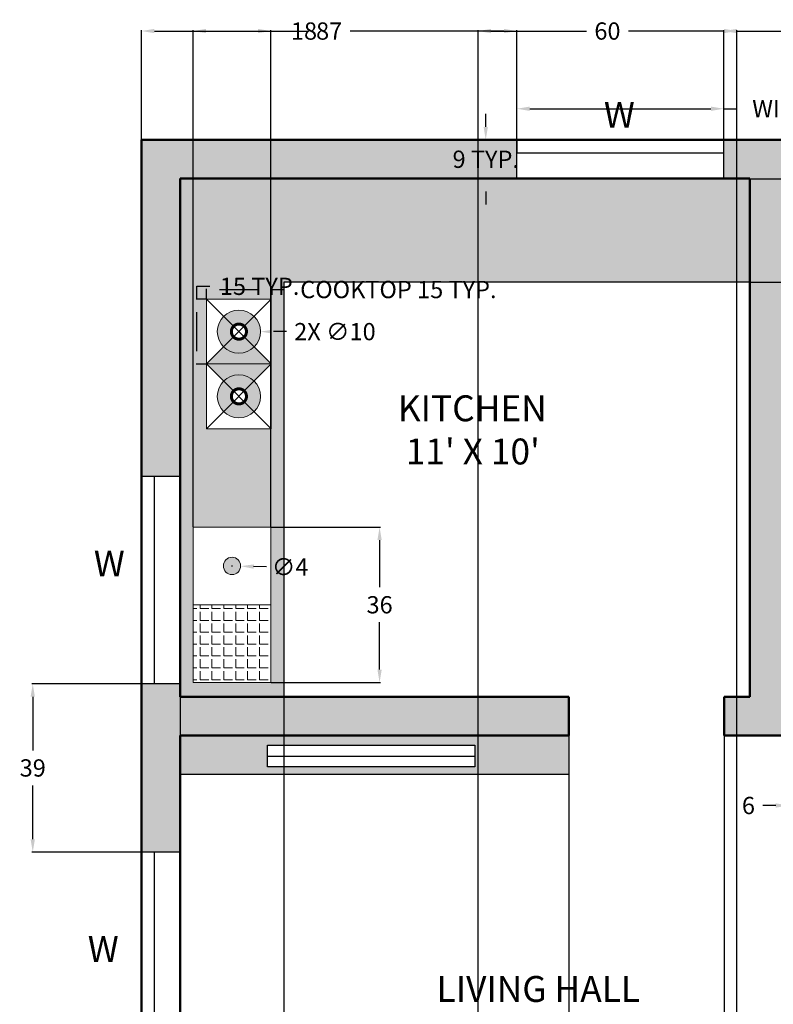
# Model space of a CAD drawing. Units: inches. Extents: x 30 to 385, y 81 to 626.
# Tile 3 of 4: x 30 to 204, y 398 to 626. Entities that reach past the tile are written whole.
import ezdxf

# ---------------------------------------------------------------- set-up
doc = ezdxf.new("R2010")
doc.units = ezdxf.units.IN
doc.header["$MEASUREMENT"] = 0
for name, color, linetype, lineweight in [('A-ANNO-DIMS', 2, 'Continuous', 18), ('A-ANNO-TEXT', 7, 'Continuous', 18), ('A-AREA-IDEN', 7, 'Continuous', 25), ('A-EQPM', 9, 'Continuous', 18), ('A-FLOR-CASE', 8, 'Continuous', 25), ('A-FLOR-CASE-PATT', 26, 'Continuous', 13), ('A-FLOR-FIXT', 8, 'Continuous', 18), ('A-FLOR-FIXT-PATT', 9, 'Continuous', 13), ('A-GLAZ', 4, 'Continuous', 25), ('A-WALL', 7, 'Continuous', 50), ('A-WALL-PATT', 32, 'Continuous', 13)]:
    doc.layers.add(name, color=color, linetype=linetype, lineweight=lineweight)
doc.styles.get("Standard").update_dxf_attribs({"font": 'arial.ttf'})
doc.dimstyles.get("Standard").update_dxf_attribs({"dimtxt": 4, "dimasz": 3, "dimexe": 0.18, "dimexo": 0.0625, "dimgap": 2, "dimtad": 0, "dimtih": 1, "dimtoh": 1, "dimdec": 0, "dimzin": 0, "dimdsep": 46, "dimlunit": 3, "dimtxsty": 'Standard', "dimcen": 0.09, "dimadec": 0, "dimazin": 0, "dimtfac": 1, "dimtdec": 0, "dimtofl": 0, "dimtmove": 0, "dimatfit": 3, "dimfxl": 1, "dimtolj": 1, "dimtzin": 0, "dimarcsym": 0})

# ---------------------------------------------------------------- blocks, each defined once
blk = doc.blocks.new('WIN-48')
for p, q in [((0, 0), (0, 9)), ((48, 0), (48, 9)), ((0, 6), (48, 6))]:
    blk.add_line(p, q)
blk = doc.blocks.new('COOKTOP-BURNER')
for p, q in [((-7.5, 7.5), (7.5, -7.5)), ((-7.5, -7.5), (7.5, 7.5))]:
    blk.add_line(p, q)
at = {"const_width": 0.7}
blk.add_lwpolyline([(-1.75, 0, 1), (1.75, 0, 1)], format="xyb", close=True, dxfattribs=at)
blk.add_circle((0, 0), 5)
blk = doc.blocks.new('*D6')
at = {"layer": 'A-ANNO-DIMS', "color": 0, "lineweight": -2, "transparency": 16777216}
for p, q in [((144.92, 598.13), (144.92, 605.44)), ((147.92, 605.26), (189.92, 605.26)), ((192.92, 598.13), (192.92, 605.44)), ((192.92, 605.26), (195.92, 605.26))]:
    blk.add_line(p, q, dxfattribs=at)
at = {"layer": 'A-ANNO-DIMS', "color": 0, "transparency": 16777216}
for points in [[(147.92, 605.76), (147.92, 604.76), (144.92, 605.26)], [(189.92, 605.76), (189.92, 604.76), (192.92, 605.26)]]:
    blk.add_solid(points, dxfattribs=at)
at = {"layer": 'Defpoints', "color": 0, "transparency": 16777216}
for p in [(192.92, 605.26), (144.92, 598.06), (192.92, 598.06)]:
    blk.add_point(p, dxfattribs=at)
at = {"layer": 'A-ANNO-DIMS', "color": 0, "transparency": 16777216, "insert": (220.77, 605.26), "char_height": 4, "attachment_point": 5}
blk.add_mtext('\\A1;WINDOW 48 TYP.', dxfattribs=at)
blk = doc.blocks.new('*D7')
at = {"layer": 'A-ANNO-DIMS', "color": 0, "lineweight": -2, "transparency": 16777216}
for p, q in [((137.72, 601.06), (137.72, 604.06)), ((144.86, 598.06), (137.54, 598.06)), ((144.86, 589.06), (137.54, 589.06)), ((137.72, 586.06), (137.72, 583.06))]:
    blk.add_line(p, q, dxfattribs=at)
at = {"layer": 'A-ANNO-DIMS', "color": 0, "transparency": 16777216}
for points in [[(137.22, 601.06), (138.22, 601.06), (137.72, 598.06)], [(137.22, 586.06), (138.22, 586.06), (137.72, 589.06)]]:
    blk.add_solid(points, dxfattribs=at)
at = {"layer": 'Defpoints', "color": 0, "transparency": 16777216}
for p in [(137.72, 598.06), (144.92, 598.06), (144.92, 589.06)]:
    blk.add_point(p, dxfattribs=at)
at = {"layer": 'A-ANNO-DIMS', "color": 0, "transparency": 16777216, "insert": (137.72, 593.56), "char_height": 4, "attachment_point": 5}
blk.add_mtext('\\A1;9 TYP.', dxfattribs=at)
blk = doc.blocks.new('*D14')
at = {"layer": 'A-ANNO-DIMS', "color": 0, "lineweight": -2, "transparency": 16777216}
for p, q in [((73, 561.2), (73, 563.56)), ((76, 563.38), (85, 563.38)), ((88, 561.2), (88, 563.56)), ((88, 563.38), (91, 563.38))]:
    blk.add_line(p, q, dxfattribs=at)
at = {"layer": 'A-ANNO-DIMS', "color": 0, "transparency": 16777216}
for points in [[(76, 563.88), (76, 562.88), (73, 563.38)], [(85, 563.88), (85, 562.88), (88, 563.38)]]:
    blk.add_solid(points, dxfattribs=at)
at = {"layer": 'Defpoints', "color": 0, "transparency": 16777216}
for p in [(88, 563.38), (73, 561.13), (88, 561.13)]:
    blk.add_point(p, dxfattribs=at)
at = {"layer": 'A-ANNO-DIMS', "color": 0, "transparency": 16777216, "insert": (117.46, 563.38), "char_height": 4, "attachment_point": 5}
blk.add_mtext('\\A1;COOKTOP 15 TYP.', dxfattribs=at)
blk = doc.blocks.new('*D15')
at = {"layer": 'A-ANNO-DIMS', "color": 0, "lineweight": -2, "transparency": 16777216}
for p, q in [((70.75, 561.13), (70.75, 564.13)), ((70.75, 564.13), (73.75, 564.13)), ((72.94, 561.13), (70.57, 561.13)), ((70.75, 549.13), (70.75, 558.13)), ((72.94, 546.13), (70.57, 546.13))]:
    blk.add_line(p, q, dxfattribs=at)
at = {"layer": 'A-ANNO-DIMS', "color": 0, "transparency": 16777216}
for points in [[(70.25, 558.13), (71.25, 558.13), (70.75, 561.13)], [(70.25, 549.13), (71.25, 549.13), (70.75, 546.13)]]:
    blk.add_solid(points, dxfattribs=at)
at = {"layer": 'Defpoints', "color": 0, "transparency": 16777216}
for p in [(70.75, 561.13), (73, 561.13), (73, 546.13)]:
    blk.add_point(p, dxfattribs=at)
at = {"layer": 'A-ANNO-DIMS', "color": 0, "transparency": 16777216, "insert": (85.3, 564.13), "char_height": 4, "attachment_point": 5}
blk.add_mtext('\\A1;15 TYP.', dxfattribs=at)
blk = doc.blocks.new('*D25')
at = {"layer": 'A-ANNO-DIMS', "color": 0, "lineweight": -2, "transparency": 16777216}
for p, q in [((57.86, 472.06), (32.54, 472.06)), ((32.72, 469.06), (32.72, 456.61)), ((32.72, 436.06), (32.72, 448.52)), ((57.86, 433.06), (32.54, 433.06))]:
    blk.add_line(p, q, dxfattribs=at)
at = {"layer": 'A-ANNO-DIMS', "color": 0, "transparency": 16777216}
for points in [[(32.22, 469.06), (33.22, 469.06), (32.72, 472.06)], [(32.22, 436.06), (33.22, 436.06), (32.72, 433.06)]]:
    blk.add_solid(points, dxfattribs=at)
at = {"layer": 'Defpoints', "color": 0, "transparency": 16777216}
for p in [(32.72, 472.06), (57.92, 472.06), (57.92, 433.06)]:
    blk.add_point(p, dxfattribs=at)
at = {"layer": 'A-ANNO-DIMS', "color": 0, "transparency": 16777216, "insert": (32.72, 452.56), "char_height": 4, "attachment_point": 5}
blk.add_mtext('\\A1;39', dxfattribs=at)
blk = doc.blocks.new('*D26')
at = {"layer": 'A-ANNO-DIMS', "color": 0, "lineweight": -2, "transparency": 16777216}
for p, q in [((57.92, 598.13), (57.92, 623.44)), ((60.92, 623.26), (96.55, 623.26)), ((141.92, 623.26), (106.29, 623.26)), ((144.92, 598.13), (144.92, 623.44))]:
    blk.add_line(p, q, dxfattribs=at)
at = {"layer": 'A-ANNO-DIMS', "color": 0, "transparency": 16777216}
for points in [[(60.92, 623.76), (60.92, 622.76), (57.92, 623.26)], [(141.92, 623.76), (141.92, 622.76), (144.92, 623.26)]]:
    blk.add_solid(points, dxfattribs=at)
at = {"layer": 'Defpoints', "color": 0, "transparency": 16777216}
for p in [(144.92, 623.26), (57.92, 598.06), (144.92, 598.06)]:
    blk.add_point(p, dxfattribs=at)
at = {"layer": 'A-ANNO-DIMS', "color": 0, "transparency": 16777216, "insert": (101.42, 623.26), "char_height": 4, "attachment_point": 5}
blk.add_mtext('\\A1;87', dxfattribs=at)
blk = doc.blocks.new('*D27')
at = {"layer": 'A-ANNO-DIMS', "color": 0, "lineweight": -2, "transparency": 16777216}
for p, q in [((192.92, 598.13), (192.92, 623.44)), ((195.92, 623.26), (207.92, 623.26)), ((210.92, 598.13), (210.92, 623.44)), ((210.92, 623.26), (213.92, 623.26))]:
    blk.add_line(p, q, dxfattribs=at)
at = {"layer": 'A-ANNO-DIMS', "color": 0, "transparency": 16777216}
for points in [[(195.92, 623.76), (195.92, 622.76), (192.92, 623.26)], [(207.92, 623.76), (207.92, 622.76), (210.92, 623.26)]]:
    blk.add_solid(points, dxfattribs=at)
at = {"layer": 'Defpoints', "color": 0, "transparency": 16777216}
for p in [(210.92, 623.26), (192.92, 598.06), (210.92, 598.06)]:
    blk.add_point(p, dxfattribs=at)
at = {"layer": 'A-ANNO-DIMS', "color": 0, "transparency": 16777216, "insert": (218.6, 623.26), "char_height": 4, "attachment_point": 5}
blk.add_mtext('\\A1;18', dxfattribs=at)
blk = doc.blocks.new('*D28')
at = {"layer": 'A-ANNO-DIMS', "color": 0, "lineweight": -2, "transparency": 16777216}
for p, q in [((66.92, 469), (66.92, 83.68)), ((90.92, 469), (90.92, 83.68)), ((69.92, 83.86), (74.03, 83.86)), ((87.92, 83.86), (83.81, 83.86))]:
    blk.add_line(p, q, dxfattribs=at)
at = {"layer": 'A-ANNO-DIMS', "color": 0, "transparency": 16777216}
for points in [[(69.92, 84.36), (69.92, 83.36), (66.92, 83.86)], [(87.92, 84.36), (87.92, 83.36), (90.92, 83.86)]]:
    blk.add_solid(points, dxfattribs=at)
at = {"layer": 'Defpoints', "color": 0, "transparency": 16777216}
for p in [(66.92, 469.06), (90.92, 469.06), (90.92, 83.86)]:
    blk.add_point(p, dxfattribs=at)
at = {"layer": 'A-ANNO-DIMS', "color": 0, "transparency": 16777216, "insert": (78.92, 83.86), "char_height": 4, "attachment_point": 5}
blk.add_mtext('\\A1;24', dxfattribs=at)
blk = doc.blocks.new('*D29')
at = {"layer": 'A-ANNO-DIMS', "color": 0, "lineweight": -2, "transparency": 16777216}
for p, q in [((198.98, 589.06), (374.3, 589.06)), ((374.12, 586.06), (374.12, 581.07)), ((374.12, 568.06), (374.12, 573.06)), ((198.98, 565.06), (374.3, 565.06))]:
    blk.add_line(p, q, dxfattribs=at)
at = {"layer": 'A-ANNO-DIMS', "color": 0, "transparency": 16777216}
for points in [[(373.62, 586.06), (374.62, 586.06), (374.12, 589.06)], [(373.62, 568.06), (374.62, 568.06), (374.12, 565.06)]]:
    blk.add_solid(points, dxfattribs=at)
at = {"layer": 'Defpoints', "color": 0, "transparency": 16777216}
for p in [(198.92, 589.06), (374.12, 589.06), (198.92, 565.06)]:
    blk.add_point(p, dxfattribs=at)
at = {"layer": 'A-ANNO-DIMS', "color": 0, "transparency": 16777216, "insert": (374.12, 577.06), "char_height": 4, "attachment_point": 5}
blk.add_mtext('\\A1;24', dxfattribs=at)
blk = doc.blocks.new('*D30')
at = {"layer": 'A-ANNO-DIMS', "color": 0, "lineweight": -2, "transparency": 16777216}
for p, q in [((69.91, 508.42), (69.91, 623.44)), ((72.91, 623.26), (84.91, 623.26)), ((87.91, 508.42), (87.91, 623.44)), ((87.91, 623.26), (90.91, 623.26))]:
    blk.add_line(p, q, dxfattribs=at)
at = {"layer": 'A-ANNO-DIMS', "color": 0, "transparency": 16777216}
for points in [[(72.91, 623.76), (72.91, 622.76), (69.91, 623.26)], [(84.91, 623.76), (84.91, 622.76), (87.91, 623.26)]]:
    blk.add_solid(points, dxfattribs=at)
at = {"layer": 'Defpoints', "color": 0, "transparency": 16777216}
for p in [(87.91, 623.26), (69.91, 508.36), (87.91, 508.36)]:
    blk.add_point(p, dxfattribs=at)
at = {"layer": 'A-ANNO-DIMS', "color": 0, "transparency": 16777216, "insert": (95.59, 623.26), "char_height": 4, "attachment_point": 5}
blk.add_mtext('\\A1;18', dxfattribs=at)
blk = doc.blocks.new('*D31')
at = {"layer": 'A-ANNO-DIMS', "color": 0, "lineweight": -2, "transparency": 16777216}
for p, q in [((87.97, 508.36), (113.29, 508.36)), ((113.11, 505.36), (113.11, 494.4)), ((113.11, 475.36), (113.11, 486.31)), ((87.97, 472.36), (113.29, 472.36))]:
    blk.add_line(p, q, dxfattribs=at)
at = {"layer": 'A-ANNO-DIMS', "color": 0, "transparency": 16777216}
for points in [[(112.61, 505.36), (113.61, 505.36), (113.11, 508.36)], [(112.61, 475.36), (113.61, 475.36), (113.11, 472.36)]]:
    blk.add_solid(points, dxfattribs=at)
at = {"layer": 'Defpoints', "color": 0, "transparency": 16777216}
for p in [(87.91, 508.36), (87.91, 472.36), (113.11, 472.36)]:
    blk.add_point(p, dxfattribs=at)
at = {"layer": 'A-ANNO-DIMS', "color": 0, "transparency": 16777216, "insert": (113.11, 490.36), "char_height": 4, "attachment_point": 5}
blk.add_mtext('\\A1;36', dxfattribs=at)
blk = doc.blocks.new('*D32')
at = {"layer": 'A-ANNO-DIMS', "color": 0, "lineweight": -2, "transparency": 16777216}
for p, q in [((135.92, 247.13), (135.92, 623.44)), ((138.92, 623.26), (161.05, 623.26)), ((192.92, 623.26), (170.79, 623.26)), ((195.92, 247.13), (195.92, 623.44))]:
    blk.add_line(p, q, dxfattribs=at)
at = {"layer": 'A-ANNO-DIMS', "color": 0, "transparency": 16777216}
for points in [[(138.92, 623.76), (138.92, 622.76), (135.92, 623.26)], [(192.92, 623.76), (192.92, 622.76), (195.92, 623.26)]]:
    blk.add_solid(points, dxfattribs=at)
at = {"layer": 'Defpoints', "color": 0, "transparency": 16777216}
for p in [(195.92, 623.26), (135.92, 247.06), (195.92, 247.06)]:
    blk.add_point(p, dxfattribs=at)
at = {"layer": 'A-ANNO-DIMS', "color": 0, "transparency": 16777216, "insert": (165.92, 623.26), "char_height": 4, "attachment_point": 5}
blk.add_mtext('\\A1;60', dxfattribs=at)
blk = doc.blocks.new('*D33')
at = {"layer": 'A-ANNO-DIMS', "color": 0, "lineweight": -2, "transparency": 16777216}
for p, q in [((156.96, 460), (156.96, 83.68)), ((192.96, 460), (192.96, 83.68)), ((159.96, 83.86), (170.09, 83.86)), ((189.96, 83.86), (179.82, 83.86))]:
    blk.add_line(p, q, dxfattribs=at)
at = {"layer": 'A-ANNO-DIMS', "color": 0, "transparency": 16777216}
for points in [[(159.96, 84.36), (159.96, 83.36), (156.96, 83.86)], [(189.96, 84.36), (189.96, 83.36), (192.96, 83.86)]]:
    blk.add_solid(points, dxfattribs=at)
at = {"layer": 'Defpoints', "color": 0, "transparency": 16777216}
for p in [(156.96, 460.06), (192.96, 460.06), (192.96, 83.86)]:
    blk.add_point(p, dxfattribs=at)
at = {"layer": 'A-ANNO-DIMS', "color": 0, "transparency": 16777216, "insert": (174.96, 83.86), "char_height": 4, "attachment_point": 5}
blk.add_mtext('\\A1;36', dxfattribs=at)
blk = doc.blocks.new('*D35')
at = {"layer": 'A-ANNO-DIMS', "color": 0, "lineweight": -2, "transparency": 16777216}
for p, q in [((207.92, 469), (207.92, 443.68)), ((213.92, 469), (213.92, 443.68)), ((204.92, 443.86), (201.92, 443.86)), ((216.92, 443.86), (219.92, 443.86))]:
    blk.add_line(p, q, dxfattribs=at)
at = {"layer": 'A-ANNO-DIMS', "color": 0, "transparency": 16777216}
for points in [[(204.92, 444.36), (204.92, 443.36), (207.92, 443.86)], [(216.92, 444.36), (216.92, 443.36), (213.92, 443.86)]]:
    blk.add_solid(points, dxfattribs=at)
at = {"layer": 'Defpoints', "color": 0, "transparency": 16777216}
for p in [(207.92, 469.06), (213.92, 469.06), (207.92, 443.86)]:
    blk.add_point(p, dxfattribs=at)
at = {"layer": 'A-ANNO-DIMS', "color": 0, "transparency": 16777216, "insert": (198.6, 443.86), "char_height": 4, "attachment_point": 5}
blk.add_mtext('\\A1;6', dxfattribs=at)
blk = doc.blocks.new('*D52')
at = {"layer": 'A-ANNO-DIMS', "color": 0, "lineweight": -2, "transparency": 16777216}
for p, q in [((78.82, 499.36), (79, 499.36)), ((78.91, 499.27), (78.91, 499.45)), ((86.9, 499.13), (83.9, 499.21))]:
    blk.add_line(p, q, dxfattribs=at)
at = {"layer": 'A-ANNO-DIMS', "color": 0, "transparency": 16777216}
blk.add_solid([(83.92, 499.71), (83.89, 498.71), (80.91, 499.3)], dxfattribs=at)
at = {"layer": 'Defpoints', "color": 0, "transparency": 16777216}
for p in [(76.91, 499.42), (80.91, 499.3)]:
    blk.add_point(p, dxfattribs=at)
at = {"layer": 'A-ANNO-DIMS', "color": 0, "transparency": 16777216, "insert": (92.38, 499.13), "char_height": 4, "attachment_point": 5}
blk.add_mtext('\\A1;∅4', dxfattribs=at)
blk = doc.blocks.new('*D53')
at = {"layer": 'A-ANNO-DIMS', "color": 0, "lineweight": -2, "transparency": 16777216}
for p, q in [((80.41, 553.63), (80.59, 553.63)), ((80.5, 553.54), (80.5, 553.72)), ((91.5, 553.63), (88.5, 553.63))]:
    blk.add_line(p, q, dxfattribs=at)
at = {"layer": 'A-ANNO-DIMS', "color": 0, "transparency": 16777216}
blk.add_solid([(88.5, 554.13), (88.5, 553.13), (85.5, 553.63)], dxfattribs=at)
at = {"layer": 'Defpoints', "color": 0, "transparency": 16777216}
for p in [(75.5, 553.63), (85.5, 553.63)]:
    blk.add_point(p, dxfattribs=at)
at = {"layer": 'A-ANNO-DIMS', "color": 0, "transparency": 16777216, "insert": (102.76, 553.63), "char_height": 4, "attachment_point": 5}
blk.add_mtext('\\A1;2X ∅10', dxfattribs=at)

msp = doc.modelspace()

# ---------------------------------------------------------------- hatches: boundary and pattern name
at = {"layer": 'A-FLOR-CASE-PATT'}
h = msp.add_hatch(color=256, dxfattribs=at)
h.paths.add_polyline_path([(198.919, 589.0638), (66.919, 589.0638), (66.919, 469.0638), (90.919, 469.0638), (90.919, 565.0638), (198.919, 565.0638)])
h.paths.add_polyline_path([(88.002, 561.1334), (88.002, 531.1334), (73.002, 531.1334), (73.002, 561.1334)], flags=16)
h.paths.add_polyline_path([(85.502, 553.6334, -0.19891237), (84.0375, 550.0979), (88.002, 546.1334), (84.0375, 542.1689, -0.19891237), (85.502, 538.6334, -1), (75.502, 538.6334, -0.19891237), (76.9665, 542.1689), (73.002, 546.1334), (76.9665, 550.0979, -0.19891237), (75.502, 553.6334, -1)], flags=0)
h.paths.add_polyline_path([(82.2476, 553.6334, -1), (78.7564, 553.6334, -1)], flags=0)
h.paths.add_polyline_path([(82.2476, 538.6334, -1), (78.7564, 538.6334, -1)], flags=0)
h.paths.add_polyline_path([(87.9068, 508.3581), (87.9068, 472.3581), (69.9068, 472.3581), (69.9068, 508.3581)], flags=16)
h.paths.add_polyline_path([(80.9068, 499.3581, -1), (76.9068, 499.3581, -1)], flags=0)
h = msp.add_hatch(color=256, dxfattribs=at)
h.paths.add_polyline_path([(156.9551, 460.0638), (66.919, 460.0638), (66.919, 451.0638), (156.9551, 451.0638)])
h.paths.add_polyline_path([(135.1556, 452.8), (87.1556, 452.8), (87.1556, 457.8), (135.1556, 457.8)], flags=16)
at = {"layer": 'A-FLOR-FIXT-PATT'}
h = msp.add_hatch(dxfattribs=at)
h.set_pattern_fill('ANGLE', color=256, scale=10)
h.set_pattern_definition([(0, (0, 0), (0, 2.75), [2, -0.75]), (90, (0, 0), (-2.75, 2e-16), [2, -0.75])])
h.paths.add_polyline_path([(87.9068, 490.3581), (69.9068, 490.3581), (69.9068, 472.3581), (87.9068, 472.3581)])
at = {"layer": 'A-WALL-PATT'}
msp.add_hatch(color=256, dxfattribs=at).paths.add_polyline_path([(144.919, 598.0638), (57.919, 598.0638), (57.919, 520.0638), (66.919, 520.0638), (66.919, 589.0638), (144.919, 589.0638)])
h = msp.add_hatch(color=256, dxfattribs=at)
h.paths.add_polyline_path([(156.9551, 469.0638), (66.919, 469.0638), (66.919, 472.0638), (57.919, 472.0638), (57.919, 433.0638), (66.919, 433.0638), (66.919, 460.0638), (156.9551, 460.0638)])
h.paths.add_polyline_path([(207.919, 589.0638), (210.919, 589.0638), (210.919, 598.0638), (192.919, 598.0638), (192.919, 589.0638), (198.919, 589.0638), (198.919, 469.0638), (192.9551, 469.0638), (192.9551, 460.0638), (213.919, 460.0638), (213.919, 469.0638), (207.919, 469.0638)])
h.paths.add_polyline_path([(348.919, 598.0638), (258.919, 598.0638), (258.919, 589.0638), (339.919, 589.0638), (339.919, 469.0638), (336.919, 469.0638), (336.919, 460.0638), (339.919, 460.0638), (339.919, 442.0638), (348.919, 442.0638)])

# ---------------------------------------------------------------- linework, layer by layer
at = {"layer": 'A-EQPM'}
for p, q in [((73.002, 546.1334), (88.002, 546.1334)), ((73.002, 531.1334), (88.002, 531.1334))]:
    msp.add_line(p, q, dxfattribs=at)
msp.add_lwpolyline([(73.002, 561.1334), (88.002, 561.1334), (88.002, 531.1334), (73.002, 531.1334)], close=True, dxfattribs=at)
at = {"layer": 'A-FLOR-CASE'}
for p, q in [((198.919, 565.0638), (90.919, 565.0638)), ((90.919, 565.0638), (90.919, 469.0638)), ((156.9551, 460.0638), (156.9551, 451.0638)), ((87.1556, 455.3), (135.1556, 455.3)), ((156.9551, 451.0638), (66.919, 451.0638))]:
    msp.add_line(p, q, dxfattribs=at)
msp.add_lwpolyline([(87.1556, 457.8), (135.1556, 457.8), (135.1556, 452.8), (87.1556, 452.8)], close=True, dxfattribs=at)
at = {"layer": 'A-FLOR-FIXT'}
for p, q in [((87.9068, 508.3581), (69.9068, 508.3581)), ((69.9068, 490.3581), (87.9068, 490.3581))]:
    msp.add_line(p, q, dxfattribs=at)
msp.add_lwpolyline([(69.9068, 508.3581), (87.9068, 508.3581), (87.9068, 472.3581), (69.9068, 472.3581)], close=True, dxfattribs=at)
msp.add_circle((78.9068, 499.3581), 2, dxfattribs=at)
at = {"layer": 'A-GLAZ'}
msp.add_line((144.919, 598.0638), (144.919, 595.0638), dxfattribs=at)
at = {"layer": 'A-WALL'}
for p, q in [((348.919, 598.0638), (57.919, 598.0638)), ((57.919, 598.0638), (57.919, 109.0638)), ((66.919, 589.0638), (66.919, 469.0638)), ((198.919, 589.0638), (66.919, 589.0638)), ((198.919, 589.0638), (198.919, 469.0638)), ((156.9551, 469.0638), (66.919, 469.0638)), ((156.9551, 469.0638), (156.9551, 460.0638)), ((198.919, 469.0638), (192.9551, 469.0638)), ((192.9551, 469.0638), (192.9551, 460.0638)), ((66.919, 460.0638), (66.919, 256.0638)), ((156.9551, 460.0638), (66.919, 460.0638)), ((213.919, 460.0638), (192.9551, 460.0638))]:
    msp.add_line(p, q, dxfattribs=at)

# ---------------------------------------------------------------- block references
at = {"layer": 'A-EQPM'}
for p in [(80.502, 553.6334), (80.502, 538.6334)]:
    msp.add_blockref('COOKTOP-BURNER', p, dxfattribs=at)
at = {"layer": 'A-GLAZ'}
msp.add_blockref('WIN-48', (144.919, 589.0638), dxfattribs=at)
for p, rotation in [((66.919, 472.0638), 89.99999999999994), ((66.919, 385.0638), 90.00000000000003)]:
    msp.add_blockref('WIN-48', p, dxfattribs=dict(at, rotation=rotation))

# ---------------------------------------------------------------- texts
at = {"layer": 'A-ANNO-TEXT', "char_height": 6, "attachment_point": 1}
for insert in [(165.0879, 606.8608), (46.8673, 502.931), (45.4665, 413.6309)]:
    msp.add_mtext_dynamic_manual_height_columns('W', width=76.086845, gutter_width=1, heights=[0], dxfattribs=dict(at, insert=insert))
at = {"layer": 'A-AREA-IDEN', "char_height": 6, "attachment_point": 1}
for s, insert in [("KITCHEN\\P 11' X 10'", (117.3433, 538.8683)), ("LIVING HALL\\P  11' X 17'", (126.3177, 404.3646))]:
    msp.add_mtext_dynamic_manual_height_columns(s, width=76.086845, gutter_width=1, heights=[0], dxfattribs=dict(at, insert=insert))

# ---------------------------------------------------------------- dimensions: what is measured, and where the dimension line sits
at = {"layer": 'A-ANNO-DIMS'}
for base, p1, p2, picture, middle in [((144.919, 623.2638), (57.919, 598.0638), (144.919, 598.0638), '*D26', (101.419, 623.2638)), ((87.9068, 623.2638), (69.9068, 508.3581), (87.9068, 508.3581), '*D30', (95.5876, 623.2638)), ((195.919, 623.2638), (135.919, 247.0638), (195.919, 247.0638), '*D32', (165.919, 623.2638)), ((210.919, 623.2638), (192.919, 598.0638), (210.919, 598.0638), '*D27', (218.5998, 623.2638)), ((90.919, 83.8638), (66.919, 469.0638), (90.919, 469.0638), '*D28', (78.919, 83.8638)), ((192.9551, 83.8638), (156.9551, 460.0638), (192.9551, 460.0638), '*D33', (174.9551, 83.8638))]:
    dim = msp.add_linear_dim(base=base, p1=p1, p2=p2, dimstyle='Standard', override={"dimdec": 0, "dimlfac": 1, "dimrnd": 0, "dimzin": 0, "dimdsep": 46, "dimlunit": 2}, dxfattribs=at)
    dim.commit()
    dim.dimension.update_dxf_attribs({"geometry": picture, "text_midpoint": middle})
for base, p1, p2, text, picture, middle in [((192.919, 605.2638), (144.919, 598.0638), (192.919, 598.0638), 'WINDOW <> TYP.', '*D6', (220.7717, 605.2638)), ((88.002, 563.3834), (73.002, 561.1334), (88.002, 561.1334), 'COOKTOP <> TYP.', '*D14', (117.4618, 563.3834))]:
    dim = msp.add_linear_dim(base=base, p1=p1, p2=p2, text=text, dimstyle='Standard', override={"dimdec": 0, "dimlfac": 1, "dimrnd": 0, "dimzin": 0, "dimdsep": 46, "dimlunit": 2}, dxfattribs=at)
    dim.commit()
    dim.dimension.update_dxf_attribs({"geometry": picture, "text_midpoint": middle})
for base, p1, p2, picture, middle in [((137.719, 598.0638), (144.919, 589.0638), (144.919, 598.0638), '*D7', (137.719, 593.5638)), ((70.752, 561.1334), (73.002, 546.1334), (73.002, 561.1334), '*D15', (85.2991, 564.1334))]:
    dim = msp.add_linear_dim(base=base, p1=p1, p2=p2, angle=90, text='<> TYP.', dimstyle='Standard', override={"dimdec": 0, "dimlfac": 1, "dimrnd": 0, "dimzin": 0, "dimdsep": 46, "dimlunit": 2}, dxfattribs=at)
    dim.commit()
    dim.dimension.update_dxf_attribs({"geometry": picture, "text_midpoint": middle})
for base, p1, p2, angle, picture, middle in [((374.119, 589.0638), (198.919, 565.0638), (198.919, 589.0638), 90, '*D29', (374.119, 577.0638)), ((113.1068, 472.3581), (87.9068, 508.3581), (87.9068, 472.3581), 270, '*D31', (113.1068, 490.3581)), ((32.719, 472.0638), (57.919, 433.0638), (57.919, 472.0638), 90, '*D25', (32.719, 452.5638)), ((207.919, 443.8638), (213.919, 469.0638), (207.919, 469.0638), 180, '*D35', (198.5984, 443.8638))]:
    dim = msp.add_linear_dim(base=base, p1=p1, p2=p2, angle=angle, dimstyle='Standard', override={"dimdec": 0, "dimlfac": 1, "dimrnd": 0, "dimzin": 0, "dimdsep": 46, "dimlunit": 2}, dxfattribs=at)
    dim.commit()
    dim.dimension.update_dxf_attribs({"geometry": picture, "text_midpoint": middle})
dim = msp.add_diameter_dim_2p(p1=(75.502, 553.6338), p2=(85.502, 553.633), text='2X <>', dimstyle='Standard', override={"dimdec": 0, "dimlfac": 1, "dimrnd": 0, "dimzin": 0, "dimdsep": 46, "dimlunit": 2}, dxfattribs=at)
dim.commit()
dim.dimension.update_dxf_attribs({"geometry": '*D53', "text_midpoint": (91.502, 553.6325), "dimtype": 163})
dim = msp.add_diameter_dim_2p(p1=(76.9076, 499.4159), p2=(80.906, 499.3004), dimstyle='Standard', override={"dimdec": 0, "dimlfac": 1, "dimrnd": 0, "dimzin": 0, "dimdsep": 46, "dimlunit": 2}, dxfattribs=at)
dim.commit()
dim.dimension.update_dxf_attribs({"geometry": '*D52', "text_midpoint": (86.9035, 499.1272), "dimtype": 163})

doc.saveas('drawing.dxf')
